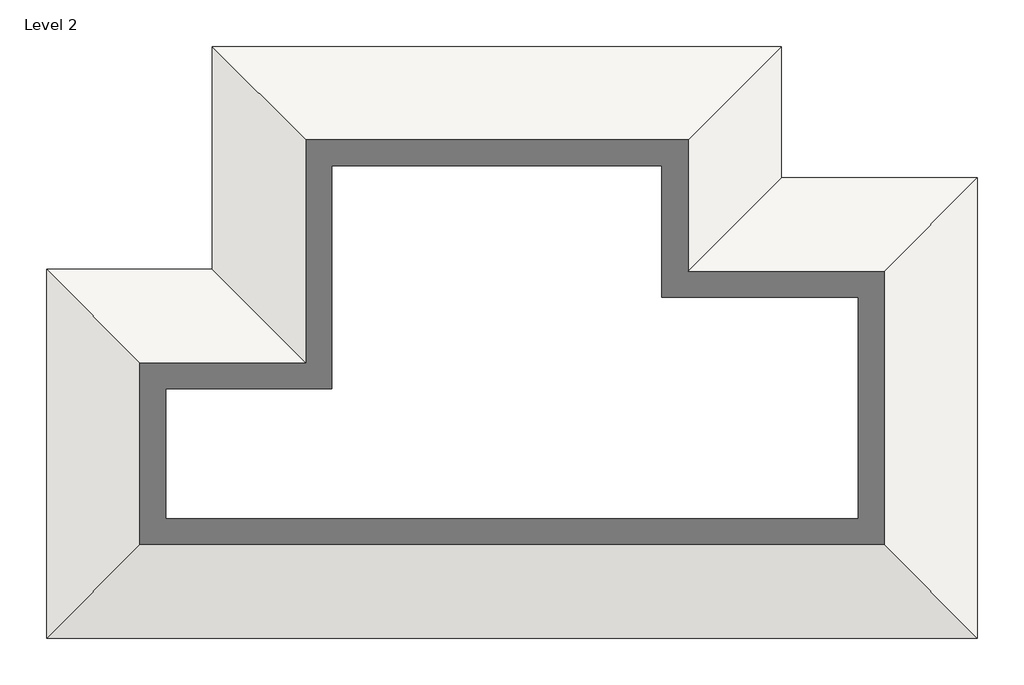
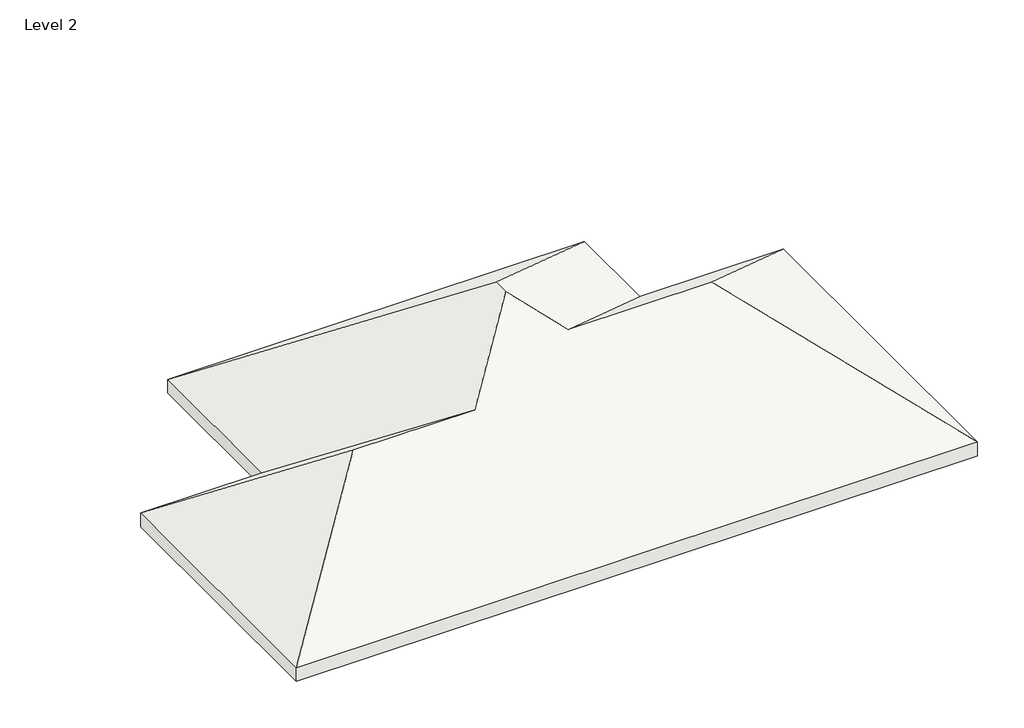
# One storey: 1 roof.
"""IFC4 building model written with IfcOpenShell, lengths in millimetres."""

from ifc_helpers import new_model, si_unit, origin, place, context, project, spatial, faceted_brep, element, save

model = new_model("IFC4")

# Units and contexts
model_context = context("Model", 3, world=origin())
ifc_project = project(units=[si_unit("LENGTHUNIT", "METRE", prefix="MILLI")], contexts=[model_context])

# Site, building, storey
site = spatial("IfcSite", under=ifc_project)
building = spatial("IfcBuilding", under=site)
storey = spatial("IfcBuildingStorey", under=building, Name="Level 2", Elevation=3048.0)

# Roof
placement = place(None, origin())
element("IfcRoof", 1, ObjectType="Wood Rafter 8\" - Asphalt Shingle - Insulated", at=placement, inside=storey, context=model_context, shape_type="Brep", body=[
    faceted_brep([(-17597.5868725, 8494.6202409, 4893.46875), (-20058.2118725, 6033.9952409, 3048.0), (-20058.2118725, 10955.2452409, 3048.0), (-7637.6118725, 6033.9952409, 3048.0), (-10707.8368725, 9104.2202409, 5350.66875), (-7637.6118725, 12174.4452409, 3048.0), (-13324.0368725, 9104.2202409, 5350.66875), (-10253.8118725, 12174.4452409, 3048.0), (-14051.1118725, 9831.2952409, 5895.975), (-14051.1118725, 10129.7452409, 5895.975), (-10253.8118725, 13927.0452409, 3048.0), (-17848.4118725, 13927.0452409, 3048.0), (-15387.7868725, 8494.6202409, 4893.46875), (-17848.4118725, 10955.2452409, 3048.0), (-20058.2118725, 6033.9952409, 3313.90625), (-17597.5868725, 8494.6202409, 5159.375), (-20058.2118725, 10955.2452409, 3313.90625), (-7637.6118725, 6033.9952409, 3313.90625), (-7637.6118725, 12174.4452409, 3313.90625), (-10707.8368725, 9104.2202409, 5616.575), (-10253.8118725, 12174.4452409, 3313.90625), (-13324.0368725, 9104.2202409, 5616.575), (-10253.8118725, 13927.0452409, 3313.90625), (-14051.1118725, 10129.7452409, 6161.88125), (-14051.1118725, 9831.2952409, 6161.88125), (-17848.4118725, 13927.0452409, 3313.90625), (-17848.4118725, 10955.2452409, 3313.90625), (-15387.7868725, 8494.6202409, 5159.375)], [[[0, 1, 2]], [[3, 4, 5]], [[5, 4, 6, 7]], [[7, 6, 8, 9, 10]], [[10, 9, 11]], [[11, 9, 8, 12, 13]], [[1, 0, 12, 8, 6, 4, 3]], [[13, 12, 0, 2]], [[14, 15, 16]], [[17, 18, 19]], [[18, 20, 21, 19]], [[20, 22, 23, 24, 21]], [[22, 25, 23]], [[25, 26, 27, 24, 23]], [[14, 17, 19, 21, 24, 27, 15]], [[26, 16, 15, 27]], [[3, 17, 14, 1]], [[5, 18, 17, 3]], [[7, 20, 18, 5]], [[10, 22, 20, 7]], [[11, 25, 22, 10]], [[13, 26, 25, 11]], [[2, 16, 26, 13]], [[1, 14, 16, 2]]]),
])

save(model, "model.ifc")

# Revit data of these elements
# Type "Wood Rafter 8\" - Asphalt Shingle - Insulated"
#   Assembly Code = "B1020"
#   Layers, outside or top first: 0' - 0 1/4" "Asphalt Shingle" (function 4); 0' - 0 5/8" "Plywood, Sheathing" (function 2); 0' - 7 1/2" "Structure, Wood Joist/Rafter Layer, Batt Insulation" (function 1)
# Element 1 (IfcRoof, "Wood Rafter 8\" - Asphalt Shingle - Insulated")
#   built-in parameter 1001705 = 20.2161 (stored number, unit not read)
#   built-in parameter 1001710 = 33615
#   Phase Created = New Construction
#   Materials on its faces: "Structure, Wood Joist/Rafter Layer, Batt Insulation", "Asphalt Shingle"
# Materials
#   "Asphalt Shingle": class "Generic", colour RGB 155 155 155, transparency 0, Description = "Asphalt roofing shingle", Cost = 0
#   "Plywood, Sheathing": class "Wood", colour RGB 212 179 113, transparency 0, Description = "Plywood, sheathing grade", Cost = 0
#   "Structure, Wood Joist/Rafter Layer, Batt Insulation": class "Wood", colour RGB 127 127 127, transparency 0, Description = "Wood framing, insulated", Cost = 0
